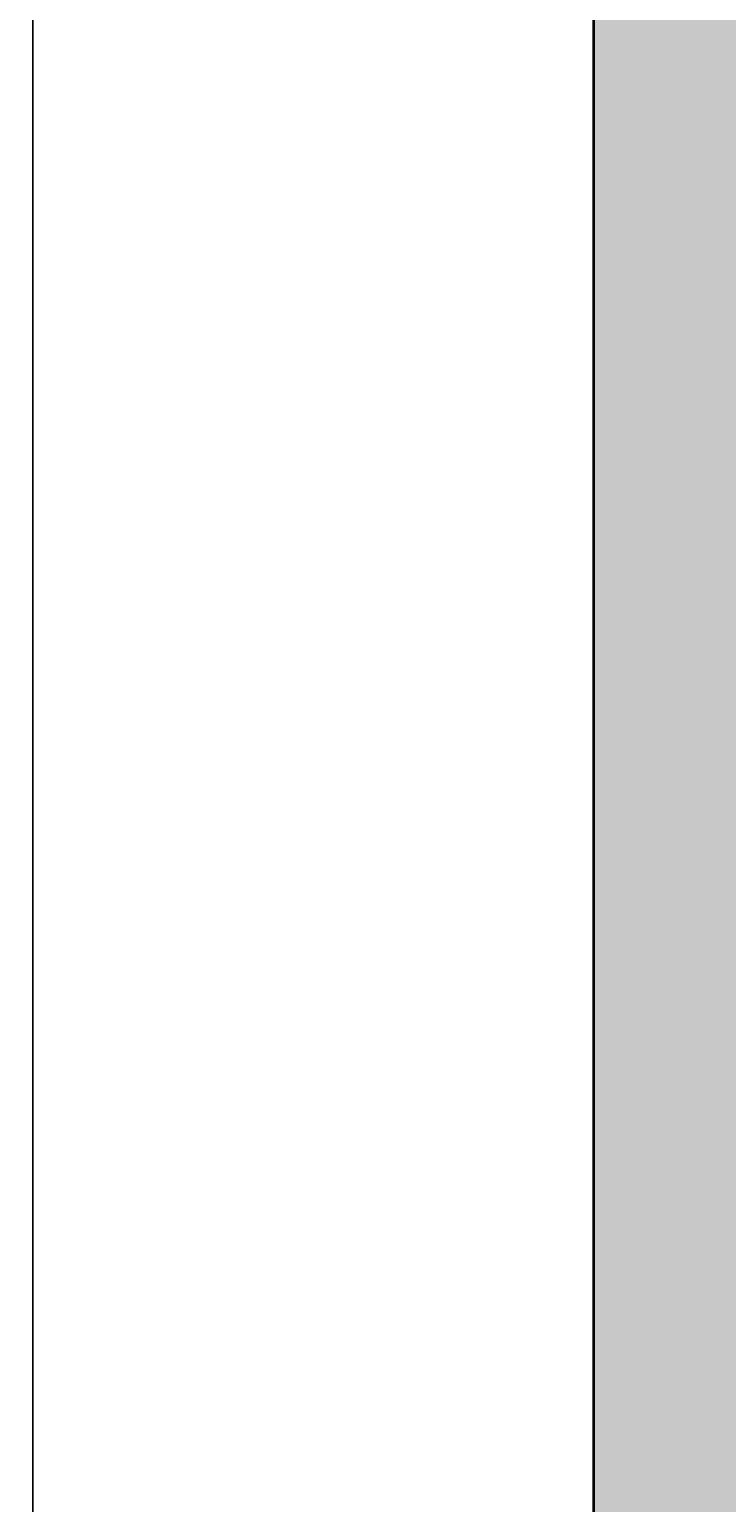
# Model space of a CAD drawing. Units: inches. Extents: x 2070 to 4408, y 1595 to 4269.
# Tile 10 of 20: x 2070 to 2111, y 2150 to 2238. Entities that reach past the tile are written whole.
import ezdxf

# ---------------------------------------------------------------- set-up
doc = ezdxf.new("R2010")
doc.units = ezdxf.units.IN
doc.layers.add('A-ANNO-DIMS', color=2, linetype='Continuous', lineweight=18)
doc.layers.add('A-WALL', color=7, linetype='Continuous', lineweight=35)
doc.layers.add('A-WALL-PATT', color=18, linetype='Continuous', lineweight=13, true_color=0x000000)
doc.styles.get("Standard").update_dxf_attribs({"font": 'arial.ttf'})
doc.dimstyles.get("Standard").update_dxf_attribs({"dimtxt": 0.18, "dimasz": 0.18, "dimexe": 0.18, "dimexo": 0.0625, "dimgap": 0.09, "dimtad": 0, "dimtih": 1, "dimtoh": 1, "dimdec": 4, "dimzin": 0, "dimdsep": 46, "dimtxsty": 'Standard', "dimcen": 0.09, "dimadec": 0, "dimazin": 0, "dimtfac": 1, "dimtdec": 4, "dimtofl": 0, "dimtmove": 0, "dimatfit": 3, "dimfxl": 1, "dimtolj": 1, "dimtzin": 0, "dimarcsym": 0})

# ---------------------------------------------------------------- blocks, each defined once
blk = doc.blocks.new('*D24')
at = {"layer": 'A-ANNO-DIMS', "color": 0, "lineweight": -2, "transparency": 16777216}
for p, q in [((2103.133, 2291.4), (2069.836, 2291.4)), ((2070.016, 2291.22), (2070.016, 1960.081)), ((2070.016, 1628.58), (2070.016, 1959.718)), ((2336.133, 1628.4), (2069.836, 1628.4))]:
    blk.add_line(p, q, dxfattribs=at)
at = {"layer": 'A-ANNO-DIMS', "color": 0, "transparency": 16777216}
for points in [[(2069.986, 2291.22), (2070.046, 2291.22), (2070.016, 2291.4)], [(2069.986, 1628.58), (2070.046, 1628.58), (2070.016, 1628.4)]]:
    blk.add_solid(points, dxfattribs=at)
at = {"layer": 'Defpoints', "color": 0, "transparency": 16777216}
for p in [(2070.016, 2291.4), (2103.196, 2291.4), (2336.196, 1628.4)]:
    blk.add_point(p, dxfattribs=at)
at = {"layer": 'A-ANNO-DIMS', "color": 0, "transparency": 16777216, "insert": (2070.016, 1959.899), "char_height": 0.18, "attachment_point": 5}
blk.add_mtext('\\A1;663', dxfattribs=at)

msp = doc.modelspace()

# ---------------------------------------------------------------- hatches: boundary and pattern name
at = {"layer": 'A-WALL-PATT'}
h = msp.add_hatch(color=256, dxfattribs=at)
h.dxf.hatch_style = 1
h.paths.add_polyline_path([(2346.196, 2218.3995), (2346.196, 2282.3995), (2340.196, 2282.3995), (2340.196, 2212.3995), (2345.5866, 2212.3995), (2346.196, 2212.3995)], flags=0)
h.paths.add_polyline_path([(2245.196, 2282.3995), (2239.196, 2282.3995), (2239.196, 2186.3995), (2244.5866, 2186.3995), (2245.196, 2186.3995)], flags=0)
h.paths.add_polyline_path([(2340.196, 2230.6455), (2245.196, 2230.6455), (2245.196, 2224.6455), (2340.196, 2224.6455)], flags=0)
h.paths.add_polyline_path([(2245.196, 2150.3995), (2239.196, 2150.3995), (2164.4362, 2150.3995), (2164.4362, 2144.3995), (2239.196, 2144.3995), (2239.196, 2086.3995), (2239.196, 2067.2711), (2244.5866, 2067.2711), (2245.196, 2067.2711), (2245.196, 2144.3995)], flags=0)
h.paths.add_polyline_path([(2346.196, 2176.3995), (2340.196, 2176.3995), (2340.196, 2086.3995), (2346.196, 2086.3995), (2346.196, 2125.318)], flags=0)
h.paths.add_polyline_path([(2446.196, 2086.3995), (2346.196, 2086.3995), (2340.196, 2086.3995), (2340.196, 2080.3995), (2446.196, 2080.3995)], flags=0)
h.paths.add_polyline_path([(2455.196, 2291.3995), (2103.196, 2291.3995), (2103.196, 1699.3995), (2336.196, 1699.3995), (2336.196, 1628.3995), (2345.196, 1628.3995), (2446.196, 1628.3995), (2454.8846, 1628.3995), (2454.8846, 1699.3995)])
h.paths.add_polyline_path([(2446.196, 2282.3995), (2446.196, 2218.3995), (2446.196, 2212.3995), (2446.196, 2086.3995), (2446.196, 2080.3995), (2446.196, 1708.3995), (2446.196, 1637.3995), (2345.196, 1637.3995), (2345.196, 1699.3995), (2345.196, 1708.3995), (2336.196, 1708.3995), (2112.196, 1708.3995), (2112.196, 2282.3995), (2239.196, 2282.3995), (2245.196, 2282.3995), (2356.196, 2282.3995)], flags=16)
h.paths.add_polyline_path([(2245.196, 2150.3995), (2245.196, 2144.3995), (2245.196, 2067.2711), (2244.5866, 2067.2711), (2239.196, 2067.2711), (2239.196, 2065.6988), (2203.2929, 2065.6988, 0.4014527), (2239.196, 2031.3337), (2244.5866, 2031.3337), (2245.196, 2031.2711), (2245.196, 1924.1525), (2239.196, 1924.1525), (2239.196, 1922.5803), (2203.2929, 1922.5803, 0.4014527), (2239.196, 1888.2151), (2244.5866, 1888.2151), (2245.196, 1888.1525), (2245.196, 1748.3995), (2339.196, 1748.4621, -0.4014527), (2303.2929, 1782.8272), (2303.2585, 1782.8272), (2303.2585, 1784.3995), (2339.196, 1784.3995), (2339.196, 1877.2067), (2291.196, 1877.2067), (2291.196, 1883.2067), (2291.196, 1946.3995), (2291.196, 1952.3995), (2291.196, 2086.3995), (2297.196, 2086.3995), (2302.196, 2086.3995), (2302.196, 2081.0259), (2303.7633, 2081.0259), (2303.7633, 2080.3995), (2338.0148, 2080.3995, 0.0043713), (2338.0203, 2081.0259), (2338.0203, 2086.3995), (2340.196, 2086.3995), (2340.196, 2176.4621), (2345.5866, 2176.4621, 0.4014527), (2381.4896, 2210.8272), (2345.5866, 2210.8272), (2345.5866, 2212.3995), (2340.196, 2212.3995), (2340.196, 2224.6455), (2245.196, 2224.6455), (2245.196, 2186.3995), (2244.5866, 2186.3995), (2239.196, 2186.3995), (2239.196, 2184.8272), (2203.2929, 2184.8272, 0.4014527), (2239.196, 2150.4621), (2244.5866, 2150.4621)], flags=0)
h.paths.add_polyline_path([(2346.196, 2282.3995), (2346.196, 2218.3995), (2377.1813, 2218.3995), (2377.1813, 2212.3995), (2346.196, 2212.3995), (2345.5866, 2212.3995), (2340.196, 2212.3995), (2340.196, 2224.6455), (2245.196, 2224.6455), (2245.196, 2230.6455), (2245.196, 2282.3995), (2292.696, 2256.5225), (2340.196, 2282.3995)], flags=0)
h.paths.add_polyline_path([(2346.196, 2086.3995), (2340.196, 2086.3995), (2340.196, 2080.3995), (2446.196, 2080.3995), (2431.196, 2016.3995), (2446.196, 1952.3995), (2412.196, 1952.3995), (2412.196, 2080.3995), (2340.196, 2080.3995), (2340.196, 2086.3995), (2340.196, 2176.3995), (2346.196, 2176.3995), (2346.196, 2125.318)], flags=0)
h.paths.add_polyline_path([(2186.508, 2270.0471, -0.0375529), (2186.9712, 2269.8581), (2186.9164, 2270.112, -0.0275912)], flags=0)
h.paths.add_polyline_path([(2183.955, 2273.7766, 1), (2188.2945, 2273.7766, 1)], flags=0)
h.paths.add_polyline_path([(2142.5261, 2274.6158, -0.0370754), (2142.5672, 2275.1696), (2142.5672, 2276.826), (2119.8759, 2276.826), (2119.8759, 2263.0962), (2140.4332, 2263.0962), (2142.5672, 2263.0962), (2142.5672, 2274.0621, -0.0370754)], flags=0)
h.paths.add_polyline_path([(2209.8974, 2263.0962), (2209.8974, 2262.2079), (2190.8042, 2262.2079), (2190.8042, 2263.0962)], flags=0)
h.paths.add_polyline_path([(2210.6382, 2276.1833), (2210.6382, 2263.9844), (2190.2185, 2263.9844), (2190.2185, 2276.1833)], flags=0)
h.paths.add_polyline_path([(2188.4362, 2273.7766, -1), (2183.8133, 2273.7766, -1)], flags=0)
h.paths.add_polyline_path([(2245.196, 2150.3995), (2245.196, 2144.3995), (2245.196, 2067.2711), (2239.196, 2067.2711), (2239.196, 2080.3995), (2172.196, 2080.3995), (2172.196, 2000.3995), (2239.196, 2000.3995), (2239.196, 1940.3995), (2159.0187, 1940.3995), (2123.0187, 1940.3995), (2112.196, 1940.3995), (2112.196, 1946.3995), (2123.0187, 1946.3995), (2123.0187, 1982.2238), (2124.586, 1982.2238), (2124.586, 1982.1895, -0.4014527), (2158.8429, 1946.3995), (2159.0187, 1946.3995), (2239.196, 1946.3995), (2239.196, 1994.3995), (2112.196, 1994.3995), (2112.196, 2000.3995), (2139.196, 2040.3995), (2112.196, 2080.3995), (2112.196, 2086.3995), (2239.196, 2086.3995), (2239.196, 2144.3995), (2209.5809, 2144.3995), (2209.5809, 2136.3995), (2203.0809, 2136.3995), (2205.0809, 2130.3996, -0.7025712), (2199.081, 2116.3995, -0.7025621), (2193.0809, 2130.3994), (2195.0809, 2136.3995), (2192.0809, 2136.3995), (2192.0809, 2134.8995), (2189.0809, 2134.8995), (2189.0809, 2135.8995), (2191.0809, 2135.8995), (2191.0809, 2136.3995), (2188.5809, 2136.3995), (2188.5809, 2144.3995), (2164.2481, 2144.3995, -0.3938585), (2130.0035, 2109.5491), (2130.0035, 2109.5147), (2128.4362, 2109.5147), (2128.4362, 2144.3995), (2112.196, 2144.3995), (2112.196, 2150.3995), (2128.4362, 2150.3995), (2128.4362, 2150.7127), (2164.4362, 2150.7127), (2164.4362, 2150.3995), (2239.196, 2150.3995)], flags=0)
h.paths.add_polyline_path([(2188.2075, 2266.8735), (2188.2075, 2211.8632, -0.4142136), (2185.4833, 2209.1391), (2146.7995, 2209.1391, -0.4142136), (2144.0754, 2211.8632), (2144.0754, 2266.8735, -0.4142136), (2146.7995, 2269.5976), (2185.4833, 2269.5976, -0.4142136)], flags=0)
h.paths.add_polyline_path([(2185.0844, 2273.7766, -1), (2187.1651, 2273.7766, -1)], flags=0)
h.paths.add_polyline_path([(2182.0486, 2259.2932), (2168.0953, 2259.2932), (2168.0953, 2260.8424), (2163.7261, 2260.8424), (2163.7261, 2259.2932), (2149.7727, 2259.2932), (2149.7727, 2266.3352), (2163.7261, 2266.3352), (2163.7261, 2261.9839), (2168.0953, 2261.9839), (2168.0953, 2266.3352), (2182.0486, 2266.3352)], flags=0)
h.paths.add_polyline_path([(2148.2585, 2250.2051), (2153.0615, 2241.8861, 0.3980705)], flags=0)
h.paths.add_polyline_path([(2162.7572, 2247.2885), (2153.1461, 2241.7396), (2148.1083, 2250.4653), (2157.7194, 2256.0142)], flags=0)
h.paths.add_polyline_path([(2162.6726, 2247.4351, -0.392862), (2157.8415, 2255.6313), (2157.6431, 2255.6313), (2157.8696, 2255.7541)], flags=0)
h.paths.add_polyline_path([(2164.2604, 2145.339), (2164.4362, 2144.3995), (2164.4362, 2150.3995), (2164.2604, 2150.7127)], flags=0)
h.paths.add_polyline_path([(2208.5809, 2142.6495), (2208.5809, 2138.3995, -0.4142136), (2207.8309, 2137.3995), (2190.5809, 2137.3995, -0.4142136), (2189.5809, 2138.1495), (2189.5809, 2142.3995, -0.4142136), (2190.3309, 2143.3995), (2207.5809, 2143.3995, -0.4142136)], flags=0)
h.paths.add_polyline_path([(2147.957, 2229.9119), (2154.7494, 2223.1195, 0.3980705)], flags=0)
h.paths.add_polyline_path([(2162.7165, 2230.8473), (2154.8691, 2222.9998), (2147.7446, 2230.1244), (2155.592, 2237.9718)], flags=0)
h.paths.add_polyline_path([(2162.5969, 2230.9669, -0.3980705), (2155.8044, 2237.7594)], flags=0)
h.paths.add_polyline_path([(2391.8776, 2049.9192), (2408.5766, 2049.9192), (2408.5766, 2033.2202), (2408.5766, 1983.123), (2408.5766, 1966.4239), (2391.8776, 1966.4239), (2391.8776, 1983.123), (2341.7804, 1983.123), (2341.7804, 2033.2202), (2391.8776, 2033.2202)], flags=0)
h.paths.add_polyline_path([(2144.1055, 2274.6158, 1), (2148.445, 2274.6158, 1)], flags=0)
h.paths.add_polyline_path([(2148.5867, 2274.6158, -1), (2143.9638, 2274.6158, -1)], flags=0)
h.paths.add_polyline_path([(2145.2349, 2274.6158, -1), (2147.3156, 2274.6158, -1)], flags=0)
edge = h.paths.add_edge_path(flags=0)
edge.add_ellipse((2400.5951, 2040.9436), major_axis=(-4.5109, 0), ratio=0.9754478, start_angle=180, end_angle=270, ccw=False)
edge.add_ellipse((2400.5951, 2040.9436), major_axis=(-4.5109, 0), ratio=0.9754478, start_angle=90, end_angle=180, ccw=False)
edge.add_ellipse((2400.5951, 2040.9436), major_axis=(-4.5109, 0), ratio=0.9754478, start_angle=0, end_angle=90, ccw=False)
edge.add_ellipse((2400.5951, 2040.9436), major_axis=(-4.5109, 0), ratio=0.9754478, start_angle=270, end_angle=360, ccw=False)
h.paths.add_polyline_path([(2199.0809, 2117.3995, -0.7345297), (2195.0809, 2130.3995), (2203.081, 2130.3995, -0.7345333)], flags=0)
h.paths.add_polyline_path([(2141.9147, 2276.0353), (2141.9147, 2263.9844), (2120.4685, 2263.9844), (2120.4685, 2276.0353)], flags=0)
h.paths.add_polyline_path([(2138.4481, 2273.4072), (2138.4481, 2266.7226), (2133.2801, 2266.7226), (2133.2801, 2273.4072)], flags=0)
h.paths.add_polyline_path([(2137.9691, 2272.9175), (2137.9691, 2272.204), (2135.4229, 2272.204), (2135.4229, 2271.6329), (2135.3221, 2270.1051), (2135.3221, 2269.0265), (2135.4229, 2268.6811), (2135.4229, 2267.2011), (2133.7212, 2267.2011), (2133.7212, 2268.6811), (2133.7983, 2269.9587), (2133.7983, 2271.2758), (2133.7212, 2271.6329), (2133.7212, 2273.0065), (2135.717, 2273.0065), (2135.717, 2272.9175)], flags=0)
h.paths.add_polyline_path([(2137.9215, 2271.8264), (2137.9215, 2271.3786), (2137.5182, 2271.3786), (2136.9355, 2271.3786), (2136.3529, 2271.3786), (2135.7703, 2271.3786), (2135.7703, 2271.8264), (2136.1736, 2271.8264), (2136.7562, 2271.8264), (2137.3389, 2271.8264)], flags=0)
h.paths.add_polyline_path([(2137.9215, 2271.692), (2137.5182, 2271.692), (2136.9355, 2271.513), (2137.3389, 2271.513)], flags=0)
h.paths.add_polyline_path([(2136.3529, 2271.692), (2135.7703, 2271.513), (2136.1736, 2271.513), (2136.7562, 2271.692)], flags=0)
h.paths.add_polyline_path([(2137.9215, 2271.513), (2137.5182, 2271.513), (2136.7562, 2271.747), (2136.7562, 2271.692), (2137.3389, 2271.692)], flags=0)
h.paths.add_polyline_path([(2137.8207, 2270.4664), (2137.8207, 2270.0971), (2137.8207, 2269.627), (2137.8207, 2269.1569), (2137.8207, 2268.6868), (2137.3837, 2268.6868), (2136.6442, 2268.6868), (2135.9271, 2268.6868), (2135.9271, 2269.0562), (2135.9271, 2269.5263), (2135.9271, 2269.9963), (2135.9271, 2270.4664), (2136.3641, 2270.4664), (2137.0812, 2270.4664)], flags=0)
h.paths.add_polyline_path([(2137.3837, 2269.627), (2137.8207, 2269.627), (2137.8207, 2269.5263), (2137.3837, 2269.5263), (2137.3837, 2269.1569), (2137.8207, 2269.1569), (2137.3837, 2269.0562), (2137.3837, 2268.6868), (2137.0812, 2268.6868), (2137.0812, 2269.0562), (2136.6442, 2269.0562), (2136.6442, 2268.6868), (2136.3641, 2268.6868), (2136.3641, 2269.0562), (2135.9271, 2269.0562), (2135.9271, 2269.1569), (2136.3641, 2269.1569), (2136.3641, 2269.5263), (2135.9271, 2269.5263), (2135.9271, 2269.627), (2136.3641, 2269.627), (2136.3641, 2269.9963), (2135.9271, 2269.9963), (2136.3641, 2270.0971), (2136.3641, 2270.4664), (2136.6442, 2270.4664), (2136.6442, 2270.0971), (2137.0812, 2270.0971), (2137.0812, 2270.4664), (2137.3837, 2270.4664), (2137.3837, 2270.0971), (2137.8207, 2270.0971), (2137.3837, 2269.9963)], flags=0)
h.paths.add_polyline_path([(2137.5182, 2271.8264), (2137.5182, 2271.692), (2137.3389, 2271.3786), (2137.3389, 2271.513)], flags=0)
h.paths.add_polyline_path([(2137.8179, 2267.8138), (2137.8179, 2267.6879), (2137.1876, 2267.6879), (2136.4733, 2267.6879), (2135.759, 2267.6879), (2135.759, 2267.8138), (2136.3893, 2267.8138), (2137.1036, 2267.8138)], flags=0)
h.paths.add_polyline_path([(2137.0812, 2269.9963), (2137.0812, 2269.627), (2137.0812, 2269.1569), (2136.6442, 2269.1569), (2136.6442, 2269.5263), (2136.6442, 2269.9963)], flags=0)
h.paths.add_polyline_path([(2136.3529, 2271.8264), (2136.3529, 2271.692), (2136.1736, 2271.3786), (2136.1736, 2271.513)], flags=0)
h.paths.add_polyline_path([(2136.4733, 2267.8138), (2136.4733, 2267.6879), (2136.3893, 2267.6879), (2136.3893, 2267.8138)], flags=0)
h.paths.add_polyline_path([(2407.9087, 2032.5522), (2407.9087, 1983.7909), (2359.81, 1983.7909, -0.0091279), (2359.0575, 1983.7909), (2342.4483, 1983.7909), (2342.4483, 2032.5522)], flags=0)
h.paths.add_polyline_path([(2389.1838, 2023.1358), (2353.7856, 2023.1358), (2353.7856, 1985.4867, -0.0921038), (2350.2788, 1988.655), (2350.2788, 2026.6426), (2389.1838, 2026.6426)], flags=0)
h.paths.add_polyline_path([(2352.6166, 2024.3048), (2351.4477, 2024.3048), (2351.4477, 2025.4737), (2352.6166, 2025.4737)], flags=0)
h.paths.add_polyline_path([(2399.6319, 2026.7589), (2404.3661, 2026.7589, -0.4142136), (2407.0379, 2024.087), (2407.0379, 2013.4908, -0.4142136), (2404.3661, 2010.819), (2399.6319, 2010.819, -0.4142136), (2396.96, 2013.4908), (2396.96, 2024.087, -0.4142136)], flags=0)
h.paths.add_polyline_path([(2399.6319, 2026.0909), (2404.3661, 2026.0909, -0.4142136), (2406.37, 2024.087), (2406.37, 2013.4908, -0.4142136), (2404.3661, 2011.487), (2399.6319, 2011.487, -0.4142136), (2397.628, 2013.4908), (2397.628, 2024.087, -0.4142136)], flags=0)
h.paths.add_polyline_path([(2399.6319, 2002.3217), (2404.3661, 2002.3217, -0.4142136), (2407.0379, 1999.6498), (2407.0379, 1989.0536, -0.4142136), (2404.3661, 1986.3818), (2399.6319, 1986.3818, -0.4142136), (2396.96, 1989.0536), (2396.96, 1999.6498, -0.4142136)], flags=0)
h.paths.add_polyline_path([(2399.6319, 2001.6537), (2404.3661, 2001.6537, -0.4142136), (2406.37, 1999.6498), (2406.37, 1989.0536, -0.4142136), (2404.3661, 1987.0497), (2399.6319, 1987.0497, -0.4142136), (2397.628, 1989.0536), (2397.628, 1999.6498, -0.4142136)], flags=0)
edge = h.paths.add_edge_path(flags=0)
edge.add_ellipse((2400.5951, 1975.3996), major_axis=(-4.5109, 0), ratio=0.9754478, start_angle=-180, end_angle=-90, ccw=False)
edge.add_ellipse((2400.5951, 1975.3996), major_axis=(-4.5109, 0), ratio=0.9754478, start_angle=90, end_angle=180, ccw=False)
edge.add_ellipse((2400.5951, 1975.3996), major_axis=(-4.5109, 0), ratio=0.9754478, start_angle=0, end_angle=90, ccw=False)
edge.add_ellipse((2400.5951, 1975.3996), major_axis=(-4.5109, 0), ratio=0.9754478, start_angle=-90, end_angle=0, ccw=False)
h.paths.add_polyline_path([(2345.196, 1910.3995), (2366.4386, 1910.3995), (2366.4386, 1925.4555), (2392.3856, 1925.4555), (2392.3856, 1933.5025), (2400.1399, 1925.4555), (2392.3856, 1919.8795), (2392.3856, 1925.4555), (2366.4386, 1925.4555), (2366.4386, 1910.3995), (2381.196, 1910.3995), (2405.196, 1910.3995), (2405.196, 1898.3995), (2446.196, 1898.3995), (2446.196, 1886.3995), (2405.196, 1886.3995), (2405.196, 1874.3995), (2446.196, 1874.3995), (2446.196, 1862.3995), (2405.196, 1862.3995), (2405.196, 1850.3995), (2446.196, 1850.3995), (2446.196, 1838.3995), (2405.196, 1838.3995), (2405.196, 1826.3995), (2446.196, 1826.3995), (2446.196, 1814.3995), (2405.196, 1814.3995), (2405.196, 1802.3995), (2446.196, 1802.3995), (2446.196, 1798.3995), (2446.196, 1792.3995), (2405.196, 1792.3995), (2405.196, 1910.3995), (2381.196, 1910.3995), (2381.196, 1792.3995), (2345.196, 1792.3995)], flags=0)
h.paths.add_polyline_path([(2333.0944, 1863.3993, -0.4142136), (2334.7225, 1861.7712), (2334.7225, 1859.329), (2335.2653, 1859.329, -0.4142136), (2337.4361, 1857.1582), (2337.4361, 1843.862, -0.4142136), (2335.2653, 1841.6911, -0.4142136), (2337.4361, 1839.5203), (2337.4361, 1827.5808, -0.4142136), (2335.2653, 1825.41, -0.4142136), (2337.4361, 1823.2392), (2337.4361, 1808.5862, -0.4142136), (2335.2653, 1806.4153), (2334.7225, 1806.4153), (2334.7225, 1803.9732, -0.4142136), (2333.0944, 1802.3451), (2317.356, 1802.3451), (2317.0846, 1802.3451, -0.4142136), (2315.7279, 1803.7018), (2315.7279, 1803.8646), (2313.8284, 1803.8646, -0.4142136), (2311.6576, 1806.0354), (2311.6576, 1823.2015, -0.395976), (2313.6834, 1825.3765, -0.433848), (2311.6576, 1827.2718), (2311.6576, 1839.761, -0.4142136), (2313.5571, 1841.6604), (2313.8284, 1841.6604), (2333.8159, 1841.6604, -0.0421362), (2334.1798, 1841.6911, -0.4142136), (2332.009, 1843.862), (2332.009, 1857.1582, -0.4142136), (2334.1798, 1859.329), (2317.356, 1859.329), (2317.0846, 1859.329, -0.4142136), (2315.7279, 1860.6858), (2315.7279, 1862.0426, -0.4142136), (2317.0846, 1863.3993), (2317.356, 1863.3993)], flags=0)
h.paths.add_polyline_path([(2208.8475, 1848.9818), (2208.8475, 1840.9741, -0.4142136), (2207.0458, 1839.1724), (2206.5453, 1839.1721), (2206.5453, 1838.7218, -0.4098586), (2204.7704, 1836.9203), (2183.7501, 1836.9203, -0.418582), (2181.9216, 1838.7218), (2181.9216, 1839.1721), (2181.421, 1839.1724, -0.4142136), (2179.6193, 1840.9741), (2179.6193, 1848.6817, -0.4406442), (2185.1126, 1854.9874), (2203.3852, 1854.9874, -0.4570796)], flags=0)
h.paths.add_polyline_path([(2204.243, 1848.4815), (2204.243, 1848.4815, 0.4172533), (2202.2204, 1850.4833), (2186.2049, 1850.4833, 0.4111805), (2184.2237, 1848.4815), (2184.2237, 1848.4815, -0.4111807), (2186.2049, 1850.4833), (2202.2204, 1850.4833, -0.4172531)], flags=0)
h.paths.add_polyline_path([(2234.7177, 1830.228), (2234.7176, 1781.6047, -0.4142136), (2233.4381, 1780.3252), (2218.6064, 1780.3252, -0.4142136), (2217.8387, 1781.0929), (2217.8387, 1783.3961, -0.4142136), (2218.6064, 1784.1639), (2218.6065, 1796.9595, -0.4142136), (2219.886, 1798.239, -0.4142136), (2218.6065, 1799.5186), (2218.6065, 1812.3142, -0.4142136), (2219.8861, 1813.5938, -0.4142136), (2218.6065, 1814.8733), (2218.6065, 1827.6689, -0.4142136), (2217.8388, 1828.4367), (2217.8388, 1830.7399, -0.4142136), (2218.6065, 1831.5076), (2233.4382, 1831.5076, -0.4142136)], flags=0)
h.paths.add_polyline_path([(2230.6344, 1827.6689, -0.4142136), (2231.4021, 1826.9012), (2231.4021, 1784.9316, -0.4142136), (2230.6343, 1784.1639), (2221.1853, 1784.1639), (2221.1853, 1827.6689)], flags=0)
h.paths.add_polyline_path([(2222.7208, 1798.239), (2221.6971, 1798.239), (2221.6971, 1813.5938), (2222.7208, 1813.5938)], flags=0)
h.paths.add_polyline_path([(2206.5453, 1773.935), (2206.5453, 1773.4848), (2206.9457, 1773.4848), (2207.0458, 1773.4845, -0.4142136), (2208.8475, 1771.6827), (2208.8475, 1763.675, -0.4422243), (2203.6505, 1757.6695), (2185.3851, 1757.6695, -0.455084), (2179.6193, 1763.9752), (2179.6193, 1771.6827, -0.4142136), (2181.421, 1773.4845), (2181.421, 1773.4848), (2181.9216, 1773.4848), (2181.9216, 1773.935, -0.4098586), (2183.6965, 1775.7366), (2204.7167, 1775.7366, -0.418582)], flags=0)
h.paths.add_polyline_path([(2202.2619, 1762.1736), (2186.2464, 1762.1736, -0.4172531), (2184.2237, 1764.1754), (2184.2237, 1764.1754, 0.4172533), (2186.2464, 1762.1736), (2202.2619, 1762.1736, 0.4111805), (2204.243, 1764.1754), (2204.243, 1764.1754, -0.4111807)], flags=0)
h.paths.add_polyline_path([(2313.0034, 1713.1906), (2312.997, 1713.1697), (2313.0123, 1713.1612)], flags=0)
h.paths.add_polyline_path([(2305.7314, 1721.0488), (2305.6257, 1721.1994), (2305.4853, 1721.084)], flags=0)
h.paths.add_polyline_path([(2307.5562, 1726.1427), (2307.6186, 1726.1026), (2307.5737, 1726.0477), (2308.5692, 1720.6434), (2310.5345, 1721.2985), (2310.5721, 1721.411), (2310.6958, 1721.3523), (2313.8453, 1722.4021), (2314.9351, 1723.8033), (2314.9294, 1723.9165), (2315.0028, 1723.8903), (2313.874, 1722.4389), (2313.8697, 1722.4102), (2308.5692, 1720.6434), (2308.9864, 1720.122), (2309.0665, 1720.0971), (2309.053, 1720.0387), (2310.9235, 1717.7005), (2311.4182, 1717.6259), (2311.2918, 1717.2402), (2312.0655, 1716.2731), (2312.1081, 1716.2606), (2312.0969, 1716.2339), (2308.5692, 1720.6434), (2305.2249, 1717.745), (2305.232, 1717.704), (2305.1665, 1717.6944), (2308.5692, 1720.6434)], flags=0)
h.paths.add_polyline_path([(2288.2072, 1714.3431), (2288.2008, 1714.3222), (2288.216, 1714.3137)], flags=0)
h.paths.add_polyline_path([(2280.9352, 1722.2013), (2280.8295, 1722.3519), (2280.689, 1722.2365)], flags=0)
h.paths.add_polyline_path([(2282.76, 1727.2952), (2282.8224, 1727.2551), (2282.7775, 1727.2002), (2283.773, 1721.7959), (2285.7383, 1722.451), (2285.7759, 1722.5635), (2285.8995, 1722.5048), (2289.0491, 1723.5546), (2290.1389, 1724.9558), (2290.1332, 1725.069), (2290.2065, 1725.0428), (2289.0777, 1723.5915), (2289.0735, 1723.5628), (2283.773, 1721.7959), (2284.1901, 1721.2745), (2284.2703, 1721.2496), (2284.2567, 1721.1913), (2286.1273, 1718.8531), (2286.622, 1718.7785), (2286.4956, 1718.3927), (2287.2692, 1717.4256), (2287.3119, 1717.4131), (2287.3006, 1717.3864), (2283.773, 1721.7959), (2280.4286, 1718.8975), (2280.4357, 1718.8565), (2280.3703, 1718.8469), (2283.773, 1721.7959)], flags=0)
h.paths.add_polyline_path([(2302.0672, 1721.8694), (2301.8205, 1721.8572), (2301.7578, 1722.1787), (2299.415, 1724.5215), (2299.103, 1724.4694), (2299.0662, 1724.8703)], flags=0)
h.paths.add_polyline_path([(2264.5643, 1715.4956), (2264.5579, 1715.4747), (2264.5731, 1715.4662)], flags=0)
h.paths.add_polyline_path([(2257.2923, 1723.3538), (2257.1865, 1723.5044), (2257.0461, 1723.389)], flags=0)
h.paths.add_polyline_path([(2259.117, 1728.4477), (2259.1795, 1728.4077), (2259.1345, 1728.3527), (2260.13, 1722.9484), (2262.0954, 1723.6036), (2262.133, 1723.716), (2262.2566, 1723.6573), (2265.4061, 1724.7071), (2266.4959, 1726.1083), (2266.4902, 1726.2215), (2266.5636, 1726.1953), (2265.4348, 1724.744), (2265.4305, 1724.7153), (2260.13, 1722.9484), (2260.5472, 1722.427), (2260.6273, 1722.4022), (2260.6138, 1722.3438), (2262.4843, 1720.0056), (2262.979, 1719.931), (2262.8526, 1719.5452), (2263.6263, 1718.5781), (2263.6689, 1718.5656), (2263.6577, 1718.5389), (2260.13, 1722.9484), (2256.7857, 1720.05), (2256.7928, 1720.009), (2256.7273, 1719.9994), (2260.13, 1722.9484)], flags=0)
h.paths.add_polyline_path([(2277.2709, 1723.0219), (2277.0243, 1723.0097), (2276.9616, 1723.3312), (2274.6187, 1725.6741), (2274.3067, 1725.6219), (2274.27, 1726.0228)], flags=0)
h.paths.add_polyline_path([(2253.628, 1724.1744), (2253.3814, 1724.1622), (2253.3186, 1724.4838), (2250.9758, 1726.8266), (2250.6638, 1726.7744), (2250.627, 1727.1753)], flags=0)
h.paths.add_polyline_path([(2161.9194, 1715.4956), (2161.913, 1715.4747), (2161.9282, 1715.4662)], flags=0)
h.paths.add_polyline_path([(2154.6474, 1723.3538), (2154.5416, 1723.5044), (2154.4012, 1723.389)], flags=0)
h.paths.add_polyline_path([(2162.7899, 1724.744), (2162.7856, 1724.7153), (2157.4851, 1722.9484), (2157.9023, 1722.427), (2157.9824, 1722.4022), (2157.9689, 1722.3438), (2159.8394, 1720.0056), (2160.3341, 1719.931), (2160.2078, 1719.5452), (2160.9814, 1718.5781), (2161.024, 1718.5656), (2161.0128, 1718.5389), (2157.4851, 1722.9484), (2154.1408, 1720.05), (2154.1479, 1720.009), (2154.0824, 1719.9994), (2157.4851, 1722.9484), (2156.4721, 1728.4477), (2156.5346, 1728.4077), (2156.4896, 1728.3527), (2157.4851, 1722.9484), (2159.4505, 1723.6036), (2159.4881, 1723.716), (2159.6117, 1723.6573), (2162.7612, 1724.7071), (2163.851, 1726.1083), (2163.8453, 1726.2215), (2163.9187, 1726.1953)], flags=0)
h.paths.add_polyline_path([(2150.9831, 1724.1744), (2150.7365, 1724.1622), (2150.6738, 1724.4838), (2148.3309, 1726.8266), (2148.0189, 1726.7744), (2147.9822, 1727.1753)], flags=0)
h.paths.add_polyline_path([(2132.5099, 1716.6482), (2132.5035, 1716.6272), (2132.5187, 1716.6187)], flags=0)
h.paths.add_polyline_path([(2125.2379, 1724.5064), (2125.1322, 1724.6569), (2124.9917, 1724.5415)], flags=0)
h.paths.add_polyline_path([(2133.3804, 1725.8965), (2133.3762, 1725.8678), (2128.0757, 1724.101), (2128.4928, 1723.5795), (2128.5729, 1723.5547), (2128.5594, 1723.4963), (2130.43, 1721.1581), (2130.9246, 1721.0835), (2130.7983, 1720.6977), (2131.5719, 1719.7306), (2131.6146, 1719.7181), (2131.6033, 1719.6914), (2128.0757, 1724.101), (2124.7313, 1721.2025), (2124.7384, 1721.1615), (2124.6729, 1721.1519), (2128.0757, 1724.101), (2127.0626, 1729.6002), (2127.1251, 1729.5602), (2127.0801, 1729.5052), (2128.0757, 1724.101), (2130.041, 1724.7561), (2130.0786, 1724.8685), (2130.2022, 1724.8098), (2133.3517, 1725.8597), (2134.4415, 1727.2608), (2134.4358, 1727.3741), (2134.5092, 1727.3478)], flags=0)
h.paths.add_polyline_path([(2121.5736, 1725.3269), (2121.327, 1725.3148), (2121.2643, 1725.6363), (2118.9214, 1727.9791), (2118.6094, 1727.9269), (2118.5727, 1728.3279)], flags=0)
h.paths.add_polyline_path([(2433.3904, 1646.406), (2433.384, 1646.3851), (2433.3992, 1646.3766)], flags=0)
h.paths.add_polyline_path([(2426.1184, 1654.2642), (2426.0127, 1654.4148), (2425.8722, 1654.2994)], flags=0)
h.paths.add_polyline_path([(2427.9432, 1659.3581), (2428.0056, 1659.318), (2427.9606, 1659.2631), (2428.9562, 1653.8588), (2430.9215, 1654.514), (2430.9591, 1654.6264), (2431.0827, 1654.5677), (2434.2323, 1655.6175), (2435.322, 1657.0187), (2435.3163, 1657.1319), (2435.3897, 1657.1057), (2434.2609, 1655.6544), (2434.2567, 1655.6257), (2428.9562, 1653.8588), (2429.3733, 1653.3374), (2429.4534, 1653.3126), (2429.4399, 1653.2542), (2431.3105, 1650.916), (2431.8051, 1650.8414), (2431.6788, 1650.4556), (2432.4524, 1649.4885), (2432.4951, 1649.476), (2432.4838, 1649.4493), (2428.9562, 1653.8588), (2425.6118, 1650.9604), (2425.6189, 1650.9194), (2425.5535, 1650.9098), (2428.9562, 1653.8588)], flags=0)
h.paths.add_polyline_path([(2376.63, 1645.4912), (2376.6236, 1645.4703), (2376.6388, 1645.4617)], flags=0)
h.paths.add_polyline_path([(2369.358, 1653.3494), (2369.2523, 1653.5), (2369.1118, 1653.3845)], flags=0)
h.paths.add_polyline_path([(2371.1828, 1658.4432), (2371.2452, 1658.4032), (2371.2003, 1658.3482), (2372.1958, 1652.944), (2374.1611, 1653.5991), (2374.1987, 1653.7116), (2374.3224, 1653.6528), (2377.4719, 1654.7027), (2378.5617, 1656.1038), (2378.556, 1656.2171), (2378.6293, 1656.1908), (2377.5005, 1654.7395), (2377.4963, 1654.7108), (2372.1958, 1652.944), (2372.6129, 1652.4225), (2372.6931, 1652.3977), (2372.6795, 1652.3393), (2374.5501, 1650.0011), (2375.0448, 1649.9265), (2374.9184, 1649.5407), (2375.692, 1648.5737), (2375.7347, 1648.5611), (2375.7234, 1648.5344), (2372.1958, 1652.944), (2368.8514, 1650.0456), (2368.8586, 1650.0046), (2368.7931, 1649.995), (2372.1958, 1652.944)], flags=0)
h.paths.add_polyline_path([(2404.0947, 1645.0338), (2404.0883, 1645.0128), (2404.1035, 1645.0043)], flags=0)
h.paths.add_polyline_path([(2396.8227, 1652.892), (2396.717, 1653.0425), (2396.5765, 1652.9271)], flags=0)
h.paths.add_polyline_path([(2398.6475, 1657.9858), (2398.7099, 1657.9458), (2398.665, 1657.8908), (2399.6605, 1652.4866), (2401.6258, 1653.1417), (2401.6634, 1653.2541), (2401.7871, 1653.1954), (2404.9366, 1654.2453), (2406.0264, 1655.6464), (2406.0207, 1655.7596), (2406.094, 1655.7334), (2404.9652, 1654.2821), (2404.961, 1654.2534), (2399.6605, 1652.4866), (2400.0776, 1651.9651), (2400.1578, 1651.9403), (2400.1442, 1651.8819), (2402.0148, 1649.5437), (2402.5095, 1649.4691), (2402.3831, 1649.0833), (2403.1567, 1648.1162), (2403.1994, 1648.1037), (2403.1881, 1648.077), (2399.6605, 1652.4866), (2396.3162, 1649.5881), (2396.3233, 1649.5471), (2396.2578, 1649.5375), (2399.6605, 1652.4866)], flags=0)
h.paths.add_polyline_path([(2419.4532, 1658.0857), (2422.4541, 1655.0848), (2422.2075, 1655.0726), (2422.1448, 1655.3941), (2419.8019, 1657.737), (2419.4899, 1657.6848)], flags=0)
h.paths.add_polyline_path([(2390.1575, 1656.7135), (2393.1584, 1653.7125), (2392.9118, 1653.7004), (2392.8491, 1654.0219), (2390.5063, 1656.3647), (2390.1943, 1656.3125)], flags=0)
h.paths.add_polyline_path([(2362.6928, 1657.1709), (2365.6937, 1654.1699), (2365.4471, 1654.1578), (2365.3844, 1654.4793), (2363.0416, 1656.8221), (2362.7295, 1656.77)], flags=0)
h.paths.add_polyline_path([(2419.9523, 2037.8601), (2440.2872, 2037.8601), (2440.2872, 2047.1732), (2419.9523, 2047.1732)], flags=8)
h.paths.add_polyline_path([(2370.186, 1698.9005), (2413.6287, 1698.9005), (2413.6287, 1708.0908), (2370.186, 1708.0908)], flags=8)
h.paths.add_polyline_path([(2370.1656, 1708.5185), (2430.0857, 1708.5185), (2430.0857, 1717.8316), (2370.1656, 1717.8316)], flags=8)
h.paths.add_polyline_path([(2254.1469, 1788.1883), (2302.2471, 1788.1883), (2302.2471, 1797.3786), (2254.1469, 1797.3786)], flags=8)
h.paths.add_polyline_path([(2254.1264, 1797.8063), (2326.1448, 1797.8063), (2326.1448, 1807.1194), (2254.1264, 1807.1194)], flags=8)
h.paths.add_polyline_path([(2300.08, 1914.5069), (2338.861, 1914.5069), (2338.861, 1923.6972), (2300.08, 1923.6972)], flags=8)
h.paths.add_polyline_path([(2300.0595, 1924.1249), (2331.5882, 1924.1249), (2331.5882, 1933.438), (2300.0595, 1933.438)], flags=8)
h.paths.add_polyline_path([(2176.6905, 1716.4567), (2224.1441, 1716.4567), (2224.1441, 1725.647), (2176.6905, 1725.647)], flags=8)
h.paths.add_polyline_path([(2176.67, 1726.0747), (2245.9176, 1726.0747), (2245.9176, 1735.3878), (2176.67, 1735.3878)], flags=8)
h.paths.add_polyline_path([(2339.997, 2039.7696), (2388.1034, 2039.7696), (2388.1034, 2048.9661), (2339.997, 2048.9661)], flags=8)
h.paths.add_polyline_path([(2339.9776, 2049.3928), (2388.7204, 2049.3928), (2388.7204, 2058.7059), (2339.9776, 2058.7059)], flags=8)
h.paths.add_polyline_path([(2366.0063, 2161.3825), (2409.449, 2161.3825), (2409.449, 2170.5728), (2366.0063, 2170.5728)], flags=8)
h.paths.add_polyline_path([(2365.9868, 2171.0016), (2405.879, 2171.0016), (2405.879, 2180.3085), (2365.9868, 2180.3085)], flags=8)
h.paths.add_polyline_path([(2366.0102, 2247.0726), (2407.12, 2247.0726), (2407.12, 2256.263), (2366.0102, 2256.263)], flags=8)
h.paths.add_polyline_path([(2365.9897, 2256.6906), (2397.9686, 2256.6906), (2397.9686, 2266.0037), (2365.9897, 2266.0037)], flags=8)
h.paths.add_polyline_path([(2271.8465, 2102.7885), (2307.6541, 2102.7885), (2307.6541, 2111.9849), (2271.8465, 2111.9849)], flags=8)
h.paths.add_polyline_path([(2271.8281, 2112.4126), (2304.2673, 2112.4126), (2304.2673, 2121.7196), (2271.8281, 2121.7196)], flags=8)
h.paths.add_polyline_path([(2141.6408, 2187.5934), (2182.108, 2187.5934), (2182.108, 2196.7837), (2141.6408, 2196.7837)], flags=8)
h.paths.add_polyline_path([(2141.6203, 2197.2114), (2190.3631, 2197.2114), (2190.3631, 2206.5245), (2141.6203, 2206.5245)], flags=8)
h.paths.add_polyline_path([(2165.7271, 2103.039), (2211.5027, 2103.039), (2211.5027, 2112.2293), (2165.7271, 2112.2293)], flags=8)
h.paths.add_polyline_path([(2165.7077, 2112.658), (2185.1033, 2112.658), (2185.1033, 2121.965), (2165.7077, 2121.965)], flags=8)
h.paths.add_polyline_path([(2174.945, 2048.0789), (2211.3973, 2048.0789), (2211.3973, 2057.2693), (2174.945, 2057.2693)], flags=8)
h.paths.add_polyline_path([(2174.9256, 2057.698), (2194.3212, 2057.698), (2194.3212, 2067.0049), (2174.9256, 2067.0049)], flags=8)
h.paths.add_polyline_path([(2164.8305, 1965.8394), (2202.9649, 1965.8394), (2202.9649, 1975.0297), (2164.8305, 1975.0297)], flags=8)
h.paths.add_polyline_path([(2164.8111, 1975.4584), (2184.2067, 1975.4584), (2184.2067, 1984.7654), (2164.8111, 1984.7654)], flags=8)
h.paths.add_polyline_path([(2133.0392, 1862.086), (2173.5065, 1862.086), (2173.5065, 1871.2763), (2133.0392, 1871.2763)], flags=8)
h.paths.add_polyline_path([(2133.0709, 1871.8585), (2157.0382, 1871.8585), (2157.0382, 1880.8585), (2133.0709, 1880.8585)], flags=8)
h.paths.add_polyline_path([(2406.4423, 1923.5541), (2418.8209, 1923.5541), (2418.8209, 1932.7199), (2406.4423, 1932.7199)], flags=8)

# ---------------------------------------------------------------- linework, layer by layer
at = {"layer": 'A-WALL'}
msp.add_lwpolyline([(2336.196, 1699.3995), (2103.196, 1699.3995), (2103.196, 2291.3995), (2455.196, 2291.3995), (2455.196, 1699.3995), (2454.8846, 1699.3995)], dxfattribs=at)

# ---------------------------------------------------------------- dimensions: what is measured, and where the dimension line sits
at = {"layer": 'A-ANNO-DIMS'}
dim = msp.add_linear_dim(base=(2070.016, 2291.3995), p1=(2336.196, 1628.3995), p2=(2103.196, 2291.3995), angle=90, dimstyle='Standard', override={"dimdec": 0, "dimlfac": 1, "dimrnd": 0, "dimzin": 0, "dimdsep": 46, "dimlunit": 2}, dxfattribs=at)
dim.commit()
dim.dimension.update_dxf_attribs({"geometry": '*D24', "text_midpoint": (2070.016, 1959.8995)})

doc.saveas('drawing.dxf')
